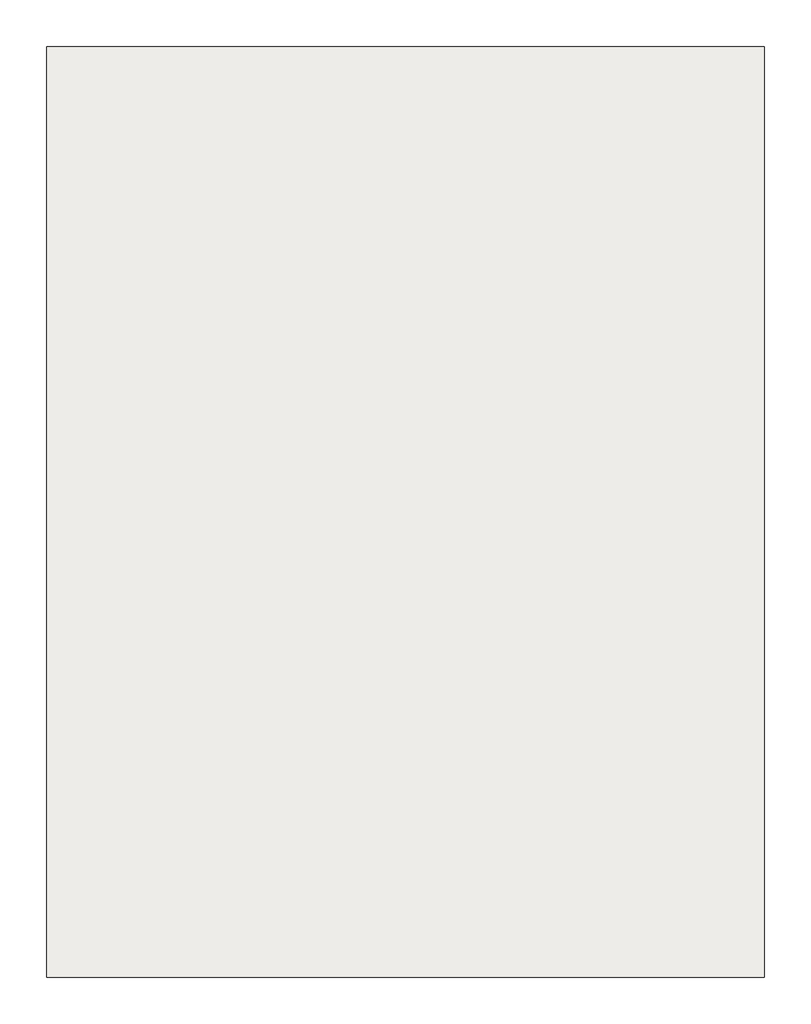
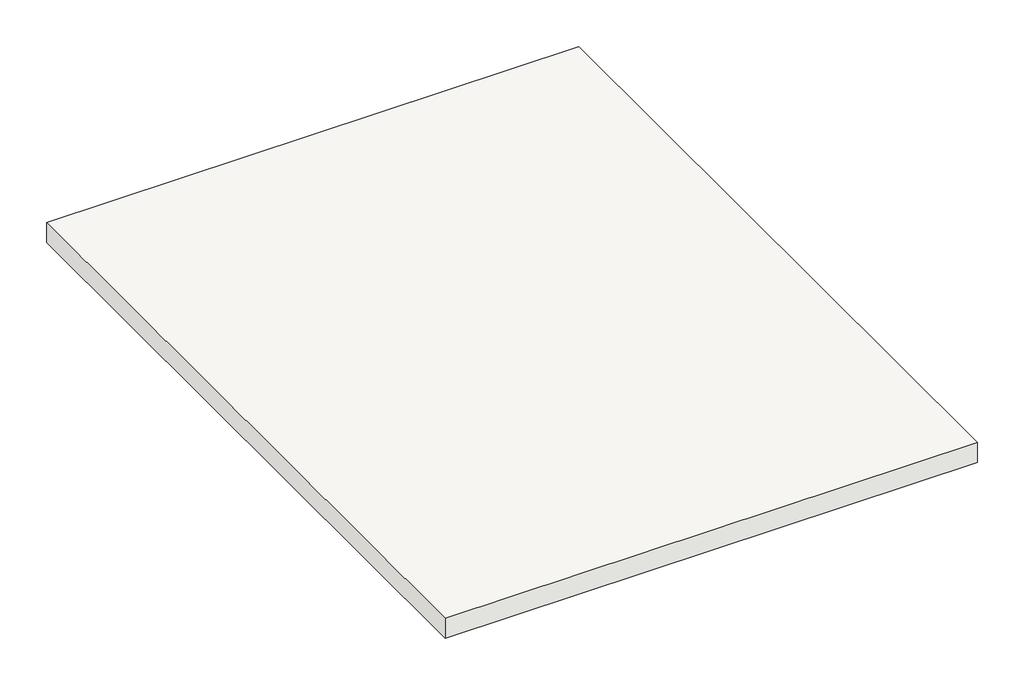
# One storey: 1 slab.
"""IFC4 building model written with IfcOpenShell, lengths in millimetres."""

from ifc_helpers import new_model, si_unit, frame, origin, place, context, project, spatial, polyline, outline, extrude, element, save

model = new_model("IFC4")

# Units and contexts
model_context = context("Model", 3, world=origin())
ifc_project = project(units=[si_unit("LENGTHUNIT", "METRE", prefix="MILLI")], contexts=[model_context])

# Site, building, storey
site = spatial("IfcSite", under=ifc_project)
building = spatial("IfcBuilding", under=site)
storey = spatial("IfcBuildingStorey", under=building, Elevation=12954.0)

# Slab
placement = place(None, origin())
element("IfcSlab", 1, at=placement, inside=storey, context=model_context, shape_type="SweptSolid", body=[
    extrude(outline(polyline([(3179.9501403, 3802.5257925), (3179.9501403, -1156.8242075), (-642.7498597, -1156.8242075), (-642.7498597, 3802.5257925), (3179.9501403, 3802.5257925)])), frame((0.0, 0.0, 12801.6), z_axis=(0.0, 0.0, 1.0), x_axis=(1.0, 0.0, 0.0)), (0.0, 0.0, 1.0), 152.4),
])

save(model, "model.ifc")

# Revit data of these elements
# Type
#   Assembly Code = "B1010"
#   Function = 0
#   Layers, outside or top first: 0' - 6" "Concrete, Cast-in-Place gray" (function 1)
# Element 1 (IfcSlab)
#   Height Offset From Level = 0' - 0"
#   Phase Created = New Construction
#   Materials on its faces: "Concrete, Cast-in-Place gray"
# Materials
#   "Concrete, Cast-in-Place gray": class "Concrete", colour RGB 192 192 192, transparency 0, Description = "Cast-in-place concrete", Cost = 0
